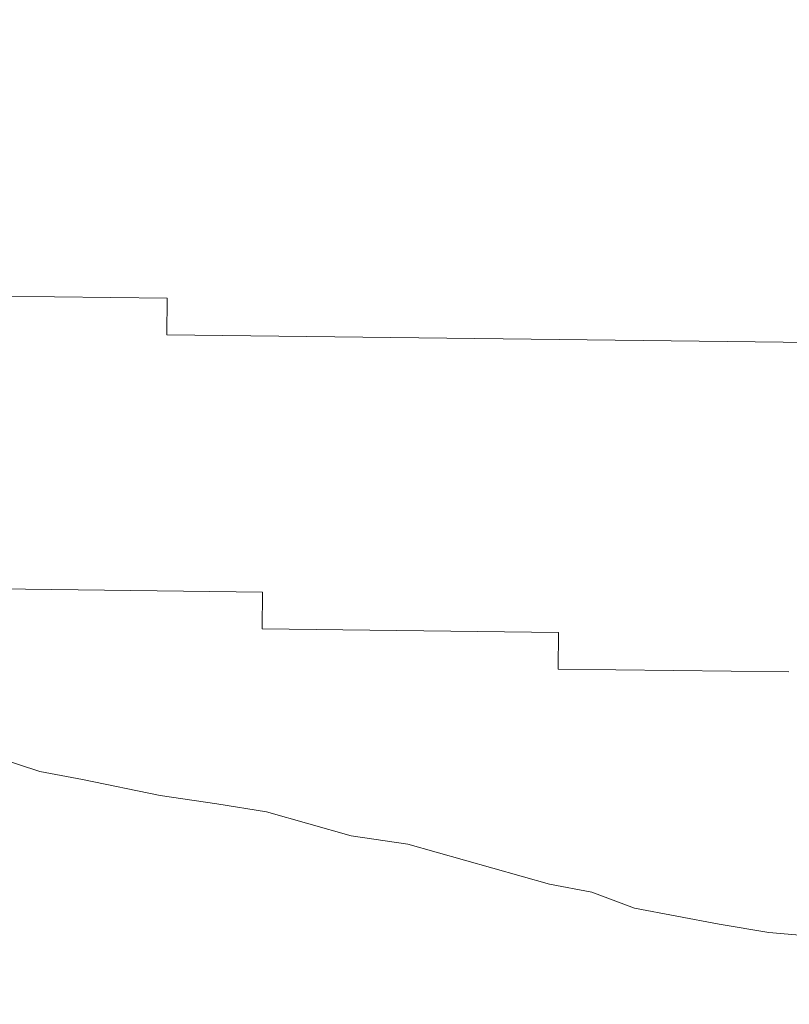
# Model space of a CAD drawing. Units: inches. Extents: x -466983 to 1020, y 324 to 318697.
# Tile 57 of 97: x 637.858 to 640.764, y 938.98 to 942.694. Entities that reach past the tile are written whole.
import ezdxf

# ---------------------------------------------------------------- set-up
doc = ezdxf.new("R2010")
doc.units = ezdxf.units.IN
doc.header["$MEASUREMENT"] = 0
doc.layers.add('A-FLOR-PATT', color=252, linetype='Continuous', lineweight=13)
doc.layers.add('A-FURN', color=8, linetype='Continuous', lineweight=18)

# ---------------------------------------------------------------- blocks, each defined once
blk = doc.blocks.new('L Shaped Sofa')
at = {"ltscale": 2}
for p, q in [((2423.7715, 750.0772), (2424.4056, 750.02)), ((2424.4056, 750.02), (2424.7468, 749.9642)), ((2424.7468, 749.9642), (2425.3317, 749.853)), ((2425.3317, 749.853), (2425.6238, 749.7432)), ((2425.6238, 749.7432), (2425.9162, 749.6876)), ((2425.9162, 749.6876), (2426.8905, 749.412)), ((2426.8905, 749.412), (2427.2805, 749.3559)), ((2427.2805, 749.3559), (2427.865, 749.1905)), ((2427.865, 749.1905), (2428.2063, 749.1347)), ((2428.2063, 749.1347), (2428.5963, 749.0787)), ((2428.5963, 749.0787), (2429.1324, 748.9677)), ((2429.1324, 748.9677), (2429.4248, 748.9121)), ((2429.4248, 748.9121), (2429.7657, 748.8021)), ((2424.2687, 748.2269), (2425.8566, 748.2075)), ((2425.8566, 748.2075), (2425.8535, 747.9556)), ((2425.8535, 747.9556), (2427.895, 747.9306)), ((2427.895, 747.9306), (2427.8919, 747.6787)), ((2427.8919, 747.6787), (2429.7066, 747.6565)), ((2423.3337, 745.9707), (2428.5509, 745.907)), ((2428.5509, 745.907), (2428.5478, 745.6551)), ((2428.5478, 745.6551), (2430.8162, 745.6274))]:
    blk.add_line(p, q, dxfattribs=at)

msp = doc.modelspace()

# ---------------------------------------------------------------- hatches: boundary and pattern name
at = {"layer": 'A-FLOR-PATT', "transparency": 33554572}
h = msp.add_hatch(dxfattribs=at)
h.set_pattern_fill('ANSI37', color=256, scale=30)
h.set_pattern_definition([(45, (-1212.4137, -290.035), (-2.6516504, 2.6516504), []), (135, (-1212.4137, -290.035), (-2.6516504, -2.6516504), [])])
h.paths.add_polyline_path([(901.8057, 1075.9377), (900.6144, 1075.9377), (900.6144, 1065.3856), (899.391, 1065.3856), (898.0911, 1065.3856), (892.8356, 1058.7098, -0.258377), (892.1875, 1058.3509), (879.9848, 1058.3509, -0.20177), (879.4382, 1058.5808), (874.0812, 1065.3856), (872.7813, 1065.3856), (871.5579, 1065.3856), (871.5579, 1075.9377), (813.8057, 1075.9377), (813.8057, 1044.7922), (832.3947, 1044.7922, -0.394795), (848.6602, 1028.5356), (848.6602, 1009.9377), (901.8057, 1009.9377), (901.8057, 1015.9377), (901.3057, 1015.9377), (871.3057, 1015.9377), (871.3057, 1017.2502), (871.3344, 1017.2502, -0.401453), (901.3057, 1045.9377), (901.8057, 1045.9377)])
edge = h.paths.add_edge_path(flags=16)
edge.add_line((847.7731, 1068.9486), (847.7731, 1073.7088))
edge.add_arc((849.2269, 1073.7088), 1.4538, 90, 180, ccw=False)
edge.add_line((849.2269, 1075.1627), (864.4921, 1075.1627))
edge.add_arc((864.4921, 1073.7088), 1.4538, 0, 90, ccw=False)
edge.add_line((865.9459, 1073.7088), (865.9459, 1069.0035))
edge.add_arc((832.6447, 1068.9761), 33.3012, -20.61234, 0.04725, ccw=False)
edge.add_ellipse((856.8595, 1058.48), major_axis=(0, 10.2131), ratio=0.6859192, start_angle=100.00884, end_angle=259.99116, ccw=False)
edge.add_arc((881.0742, 1068.9761), 33.3012, 180.04725, 200.61234, ccw=False)
h.paths.add_polyline_path([(853.1456, 1066.4815), (853.1456, 1066.4534), (853.1463, 1066.4534, 0.433107), (852.9166, 1066.6849), (852.9166, 1066.4534), (853.1456, 1066.4534), (853.1456, 1066.4815), (853.088, 1066.6122, 0.697939), (852.6995, 1066.4534), (852.7003, 1066.4534), (852.7003, 1066.4815), (852.9166, 1067.0012), (852.9166, 1066.6849, -0.396254)], flags=0)
h.paths.add_polyline_path([(861.0187, 1066.4815), (861.0187, 1066.4534), (861.0194, 1066.4534, 0.416404), (860.8024, 1066.6849), (860.8024, 1066.4534), (861.0187, 1066.4534), (861.0187, 1066.4815), (860.9672, 1066.6053, 0.713344), (860.5726, 1066.4534), (860.5734, 1066.4534), (860.5734, 1066.4815), (860.8024, 1067.0012), (860.8024, 1066.6849, -0.379973)], flags=0)
edge = h.paths.add_edge_path(flags=0)
edge.add_spline(control_points=[(861.1298, 1065.7855), (861.4661, 1065.2478), (861.6134, 1065.0161), (861.9833, 1064.3736), (862.1924, 1063.9443), (862.5614, 1063.0391), (862.7212, 1062.5633), (862.9865, 1061.5781), (863.092, 1061.0689), (863.2452, 1060.031), (863.293, 1059.5025), (863.3295, 1058.4409), (863.3181, 1057.9078), (863.2366, 1056.8518), (863.1664, 1056.3289), (862.9695, 1055.308), (862.8427, 1054.8099), (862.5365, 1053.8522), (862.3571, 1053.3927), (861.9514, 1052.5249), (861.7251, 1052.1166), (861.233, 1051.3622), (860.9672, 1051.0162), (860.4048, 1050.3949), (860.1082, 1050.1197), (859.4937, 1049.6461), (859.1758, 1049.4476), (858.5276, 1049.1299), (858.1973, 1049.0107), (857.5315, 1048.8518), (857.1959, 1048.8121), (856.5249, 1048.812), (856.1894, 1048.8515), (855.5236, 1049.0101), (855.1933, 1049.1291), (854.545, 1049.4465), (854.2271, 1049.6449), (853.6124, 1050.1183), (853.3158, 1050.3933), (852.7533, 1051.0143), (852.4874, 1051.3602), (851.9952, 1052.1144), (851.7688, 1052.5225), (851.3629, 1053.3902), (851.1834, 1053.8496), (850.877, 1054.8071), (850.7501, 1055.3051), (850.553, 1056.326), (850.4827, 1056.8488), (850.401, 1057.9048), (850.3895, 1058.4379), (850.4257, 1059.4995), (850.4734, 1060.0281), (850.6265, 1061.066), (850.7318, 1061.5753), (850.9969, 1062.5605), (851.1567, 1063.0365), (851.5254, 1063.9418), (851.7345, 1064.3712), (852.1056, 1065.0164), (852.2544, 1065.2503), (852.6082, 1065.7335)], knot_values=[3.915332, 3.915332, 3.915332, 3.915332, 4.013468, 4.013468, 4.175532, 4.175532, 4.337596, 4.337596, 4.49966, 4.49966, 4.661724, 4.661724, 4.823788, 4.823788, 4.985852, 4.985852, 5.147916, 5.147916, 5.30998, 5.30998, 5.472044, 5.472044, 5.634109, 5.634109, 5.796173, 5.796173, 5.958237, 5.958237, 6.120301, 6.120301, 6.282365, 6.282365, 6.444429, 6.444429, 6.606493, 6.606493, 6.768557, 6.768557, 6.930621, 6.930621, 7.092685, 7.092685, 7.254749, 7.254749, 7.416813, 7.416813, 7.578878, 7.578878, 7.740942, 7.740942, 7.903006, 7.903006, 8.06507, 8.06507, 8.227134, 8.227134, 8.389198, 8.389198, 8.551262, 8.551262, 8.65037, 8.65037, 8.65037, 8.65037], degree=3, periodic=0)
edge.add_line((852.6421, 1065.7855), (861.1298, 1065.7855))
edge = h.paths.add_edge_path(flags=0)
edge.add_ellipse((856.8496, 1057.7432), major_axis=(0, 7.7921), ratio=0.687861, start_angle=0, end_angle=360)
h.paths.add_polyline_path([(848.8634, 1069.3891), (848.8634, 1073.9605, -0.414214), (849.9538, 1075.0508), (863.7652, 1075.0508, -0.414214), (864.8555, 1073.9605), (864.8555, 1069.3891, -0.388936), (864.5237, 1069.027, -0.043561), (849.1953, 1069.027, -0.388936)], flags=0)
h.paths.add_polyline_path([(853.1006, 1068.1122, -1), (852.6775, 1068.1122, -1)], flags=0)
edge = h.paths.add_edge_path(flags=0)
edge.add_ellipse((856.8595, 1057.3378), major_axis=(0, 2.207), ratio=0.657164, start_angle=0, end_angle=360)
h.paths.add_polyline_path([(861.0415, 1068.1122, -1), (860.6184, 1068.1122, -1)], flags=0)
edge = h.paths.add_edge_path()
edge.add_line((573.9537, 1057.3412), (573.9537, 1075.9377))
edge.add_line((573.9537, 1075.9377), (558.7308, 1075.9377))
edge.add_line((558.7308, 1075.9377), (558.7308, 1065.3856))
edge.add_line((558.7308, 1065.3856), (557.5074, 1065.3856))
edge.add_line((557.5074, 1065.3856), (556.2075, 1065.3856))
edge.add_line((556.2075, 1065.3856), (550.952, 1058.7098))
edge.add_arc((550.3039, 1059.1155), 0.7646, 270, 327.9483, ccw=False)
edge.add_line((550.3039, 1058.3509), (538.1012, 1058.3509))
edge.add_arc((538.1012, 1059.1155), 0.7646, 224.3704, 270, ccw=False)
edge.add_line((537.5546, 1058.5808), (532.1976, 1065.3856))
edge.add_line((532.1976, 1065.3856), (530.8977, 1065.3856))
edge.add_line((530.8977, 1065.3856), (529.6743, 1065.3856))
edge.add_line((529.6743, 1065.3856), (529.6743, 1075.9377))
edge.add_line((529.6743, 1075.9377), (520.8057, 1075.9377))
edge.add_line((520.8057, 1075.9377), (520.8057, 1045.9377))
edge.add_line((520.8057, 1045.9377), (521.3057, 1045.9377))
edge.add_arc((521.3057, 1015.9377), 30, 2.50749, 90, ccw=False)
edge.add_line((551.277, 1017.2502), (551.3057, 1017.2502))
edge.add_line((551.3057, 1017.2502), (551.3057, 1015.9377))
edge.add_line((551.3057, 1015.9377), (520.8057, 1015.9377))
edge.add_line((520.8057, 1015.9377), (520.8057, 1009.9377))
edge.add_line((520.8057, 1009.9377), (559.1913, 1010.4022))
edge.add_arc((559.1913, 1011.856), 1.4538, 180, 270, ccw=False)
edge.add_line((557.7375, 1011.856), (557.7375, 1016.5613))
edge.add_arc((591.0386, 1016.5888), 33.3012, 159.38766, 180.04725, ccw=False)
edge.add_ellipse((566.8239, 1027.0848), major_axis=(0, 10.2131), ratio=0.6859192, start_angle=280.00884, end_angle=439.99116, ccw=False)
edge.add_arc((542.6091, 1016.5888), 33.3012, 0.04725, 20.61234, ccw=False)
edge.add_line((575.9103, 1016.6162), (575.9103, 1011.856))
edge.add_arc((574.4565, 1011.856), 1.4538, -90, 0, ccw=False)
edge.add_line((574.4565, 1010.4022), (608.8057, 1009.9377))
edge.add_line((608.8057, 1009.9377), (608.8057, 1041.0857))
edge.add_line((608.8057, 1041.0857), (590.2179, 1041.0857))
edge.add_arc((590.775, 1057.9074), 16.8309, 181.92775, 268.10321, ccw=False)
edge = h.paths.add_edge_path()
edge.add_ellipse((494.2443, 583.6204), major_axis=(0, 10.2131), ratio=0.6859192, start_angle=280.00884, end_angle=439.99116, ccw=False)
edge.add_arc((470.0296, 573.1243), 33.3012, 0.04725, 20.61234, ccw=False)
edge.add_line((503.3307, 573.1518), (503.3307, 568.3916))
edge.add_arc((501.8769, 568.3916), 1.4538, -90, 0, ccw=False)
edge.add_line((501.8769, 566.9377), (539.8057, 566.9377))
edge.add_line((539.8057, 566.9377), (539.8057, 572.9377))
edge.add_line((539.8057, 572.9377), (539.3057, 572.9377))
edge.add_line((539.3057, 572.9377), (509.3057, 572.9377))
edge.add_line((509.3057, 572.9377), (509.3057, 574.2502))
edge.add_line((509.3057, 574.2502), (509.3344, 574.2502))
edge.add_arc((539.3057, 572.9377), 30, 90, 177.49251, ccw=False)
edge.add_line((539.3057, 602.9377), (539.8057, 602.9377))
edge.add_line((539.8057, 602.9377), (539.8057, 626.9377))
edge.add_line((539.8057, 626.9377), (531.7718, 626.9377))
edge.add_line((531.7718, 626.9377), (531.7718, 616.3856))
edge.add_line((531.7718, 616.3856), (530.5484, 616.3856))
edge.add_line((530.5484, 616.3856), (529.2485, 616.3856))
edge.add_line((529.2485, 616.3856), (523.7105, 609.3509))
edge.add_line((523.7105, 609.3509), (510.7766, 609.3509))
edge.add_line((510.7766, 609.3509), (505.2386, 616.3856))
edge.add_line((505.2386, 616.3856), (503.9387, 616.3856))
edge.add_line((503.9387, 616.3856), (502.7153, 616.3856))
edge.add_line((502.7153, 616.3856), (502.7153, 626.9377))
edge.add_line((502.7153, 626.9377), (481.6983, 626.9377))
edge.add_line((481.6983, 626.9377), (481.6983, 610.995))
edge.add_arc((467.2703, 611.4728), 14.4359, 271.92775, 358.10321, ccw=False)
edge.add_line((467.7559, 597.0451), (451.8057, 597.0451))
edge.add_line((451.8057, 597.0451), (451.8057, 584.4035))
edge.add_line((451.8057, 584.4035), (451.8057, 566.9377))
edge.add_line((451.8057, 566.9377), (486.6117, 566.9377))
edge.add_arc((486.6117, 568.3916), 1.4538, 180, 270, ccw=False)
edge.add_line((485.1579, 568.3916), (485.1579, 573.0969))
edge.add_arc((518.4591, 573.1243), 33.3012, 159.38766, 180.04725, ccw=False)
h.paths.add_polyline_path([(836.2609, 1020.7328), (879.8898, 1020.7328), (879.8898, 1039.3902), (836.2609, 1039.3902)], flags=25)
h.paths.add_polyline_path([(549.9851, 1036.7492), (593.614, 1036.7492), (593.614, 1055.4065), (549.9851, 1055.4065)], flags=24)
h.paths.add_polyline_path([(475.123, 595.5959), (518.752, 595.5959), (518.752, 614.2532), (475.123, 614.2532)], flags=24)
h = msp.add_hatch(dxfattribs=at)
h.set_pattern_fill('ANSI37', color=256, scale=20)
h.set_pattern_definition([(45, (-1212.4137, -290.035), (-1.767767, 1.767767), []), (135, (-1212.4137, -290.035), (-1.767767, -1.767767), [])])
h.paths.add_polyline_path([(809.8057, 870.9377), (809.8057, 888.1519), (806.9985, 888.1519), (802.6624, 888.1519), (789.3832, 888.1519), (786.2846, 888.1519, -0.414214), (785.4991, 888.9374), (785.4991, 900.1959), (785.4991, 908.4696, -0.414214), (786.8082, 909.7787, -0.414214), (785.4991, 911.0878), (785.4991, 929.1015, -0.414214), (786.8082, 930.4106, -0.414214), (785.4991, 931.7197), (785.4991, 931.9039, -0.414214), (784.19, 930.5948), (766.7223, 930.5948, -0.412359), (765.4132, 931.8956, -0.413741), (764.1145, 930.5782), (744.5781, 930.422, -0.416556), (743.7864, 931.2075), (743.7864, 933.5153), (742.2154, 933.5153), (742.2154, 952.024, -0.001344), (743.7864, 952.1998), (743.7864, 953.9377), (678.5915, 953.9377), (678.5915, 951.1305), (678.5915, 946.7945), (678.5915, 933.5153), (678.5915, 930.4166, -0.414214), (677.806, 929.6312), (666.5475, 929.6312), (658.2738, 929.6312, -0.414214), (656.9647, 930.9403, -0.414214), (655.6556, 929.6312), (637.6419, 929.6312, -0.414214), (636.3328, 930.9403, -0.414214), (635.0237, 929.6312), (634.8395, 929.6312, -0.414214), (636.1486, 928.322), (636.1486, 910.8544, -0.412359), (634.8478, 909.5452, -0.413741), (636.1653, 908.2466), (636.3214, 888.7102, -0.416556), (635.5359, 887.9184), (633.2281, 887.9184), (633.2281, 886.3475), (614.7194, 886.3475, -0.001344), (614.5436, 887.9184), (612.8057, 887.9184), (612.8057, 834.9377), (612.8057, 752.9377), (612.8057, 748.9377), (612.8057, 697.9377), (654.8057, 697.9377), (654.8057, 701.9377), (715.8057, 701.9377), (715.8057, 737.4353), (774.2918, 737.4353), (774.2918, 795.9377), (809.8057, 795.9377)])
h.paths.add_polyline_path([(679.2761, 849.5757, 0.102523), (682.1475, 849.2608, -0.080461), (694.5428, 849.7725, -0.283899), (694.4822, 849.0082, 0.136605), (694.4068, 848.8103, -0.030441), (694.5428, 846.8929), (694.5428, 842.6198), (694.5428, 838.3466, -0.028219), (694.4246, 836.5684), (694.425, 836.5684, 0.196187), (694.4456, 836.2708, -0.302897), (694.5428, 835.467, -0.080461), (682.1475, 835.9787, 0.102523), (679.2761, 835.6638, -0.58611), (678.6457, 836.0169), (678.6457, 849.2227, -0.58611)], flags=16)
h.paths.add_polyline_path([(679.5173, 848.6515, 0.699597), (679.476, 848.6342, 1.20716), (679.1935, 848.7422, 0.010621)], flags=0)
h.paths.add_polyline_path([(679.4923, 836.5608, -0.013798), (679.9178, 836.6594, -0.071703), (682.8533, 837.1434, -0.165743), (682.1665, 839.1006), (682.1665, 842.6094), (682.1665, 846.0603, -0.240616), (683.4733, 848.6767, -0.068263), (693.9295, 849.0082), (693.7875, 848.7083), (693.7875, 849.0228, 0.067332), (683.4733, 848.6767, 0.240616), (682.1665, 846.0603), (682.1665, 842.6094), (682.1665, 839.1006, 0.23459), (683.461, 836.5513, 0.068093), (693.7875, 836.1955), (693.7875, 836.5104), (693.9296, 836.2102, -0.077215), (682.2421, 836.7815, 0.086627), (679.5283, 836.5701, -0.628402), (679.5029, 836.5735), (679.5029, 836.6071, 0.910458)], flags=0)
h.paths.add_polyline_path([(679.476, 848.6364), (679.2069, 848.647), (679.2069, 836.5718, 0.913566), (679.3645, 836.5861), (679.476, 836.5824)], flags=0)
h.paths.add_polyline_path([(679.2761, 829.8604, 0.102523), (682.1475, 829.5455, -0.080461), (694.5428, 830.0572, -0.283899), (694.4822, 829.2929, 0.136605), (694.4068, 829.095, -0.030441), (694.5428, 827.1776), (694.5428, 822.9045), (694.5428, 818.6314, -0.028219), (694.4246, 816.8531), (694.425, 816.8532, 0.196187), (694.4456, 816.5555, -0.302897), (694.5428, 815.7517, -0.080461), (682.1475, 816.2635, 0.102523), (679.2761, 815.9485, -0.58611), (678.6457, 816.3016), (678.6457, 829.5074, -0.58611)], flags=16)
h.paths.add_polyline_path([(679.5173, 828.9362, 0.699597), (679.476, 828.9189, 1.20716), (679.1935, 829.0269, 0.010621)], flags=0)
h.paths.add_polyline_path([(679.4923, 816.8456, -0.013798), (679.9178, 816.9441, -0.071703), (682.8533, 817.4281, -0.165743), (682.1665, 819.3853), (682.1665, 822.8941), (682.1665, 826.345, -0.240616), (683.4733, 828.9614, -0.068263), (693.9295, 829.2929), (693.7875, 828.9931), (693.7875, 829.3076, 0.067332), (683.4733, 828.9614, 0.240616), (682.1665, 826.345), (682.1665, 822.8941), (682.1665, 819.3853, 0.23459), (683.461, 816.836, 0.068093), (693.7875, 816.4802), (693.7875, 816.7952), (693.9296, 816.4949, -0.077215), (682.2421, 817.0662, 0.086627), (679.5283, 816.8549, -0.628402), (679.5029, 816.8582), (679.5029, 816.8918, 0.910458)], flags=0)
h.paths.add_polyline_path([(679.476, 828.9211), (679.2069, 828.9317), (679.2069, 816.8565, 0.913566), (679.3645, 816.8708), (679.476, 816.8671)], flags=0)
h.paths.add_polyline_path([(679.2761, 810.1451, 0.102523), (682.1475, 809.8302, -0.080461), (694.5428, 810.342, -0.3023), (694.4466, 809.5394, 0.10023), (694.4058, 809.3878, -0.03057), (694.5428, 807.4623), (694.5428, 803.1892), (694.5428, 798.9161, -0.03057), (694.4058, 796.9906, 0.10023), (694.4466, 796.839, -0.3023), (694.5428, 796.0365, -0.080461), (682.1475, 796.5482, 0.102523), (679.2761, 796.2333, -0.58611), (678.6457, 796.5863), (678.6457, 809.7921, -0.58611)], flags=16)
h.paths.add_polyline_path([(679.5173, 809.2417, 0.699597), (679.476, 809.2244, 1.20716), (679.1935, 809.3324, 0.010621)], flags=0)
h.paths.add_polyline_path([(679.4923, 797.151, -0.013798), (679.9178, 797.2496, -0.071703), (682.8533, 797.7336, -0.165743), (682.1665, 799.6908), (682.1665, 803.1996), (682.1665, 806.6505, -0.239349), (683.461, 809.2577, -0.072465), (694.4468, 809.5405, 0.197932), (694.425, 809.2405), (693.7875, 809.2985), (693.7875, 809.6135, 0.068093), (683.461, 809.2577, 0.239349), (682.1665, 806.6505), (682.1665, 803.1996), (682.1665, 799.6908, 0.235854), (683.4733, 797.1323, 0.067332), (693.7875, 796.7861), (693.7875, 797.1006), (694.425, 797.1586, 0.197932), (694.4468, 796.8586, -0.080419), (682.1557, 797.3795, 0.083867), (679.5283, 797.1603, -0.628402), (679.5029, 797.1637), (679.5029, 797.1973, 0.910458)], flags=0)
h.paths.add_polyline_path([(679.2069, 809.2372), (679.2069, 797.162, 0.913566), (679.3645, 797.1763), (679.476, 797.1726), (679.476, 809.2266)], flags=0)
h.paths.add_polyline_path([(695.3643, 853.2989), (728.2231, 853.2989), (728.2231, 771.1519), (695.3643, 771.1519)], flags=16)
h.paths.add_polyline_path([(696.0215, 852.6417), (727.5659, 852.6417), (727.5659, 771.809), (696.0215, 771.809)], flags=0)
h.paths.add_polyline_path([(679.2761, 788.7869, 0.102523), (682.1475, 788.472, -0.080461), (694.5428, 788.9837, -0.3023), (694.4466, 788.1812, 0.10023), (694.4058, 788.0296, -0.03057), (694.5428, 786.1041), (694.5428, 781.831), (694.5428, 777.5578, -0.03057), (694.4058, 775.6323, 0.10023), (694.4466, 775.4808, -0.3023), (694.5428, 774.6782, -0.080461), (682.1475, 775.19, 0.102523), (679.2761, 774.875, -0.58611), (678.6457, 775.2281), (678.6457, 788.4339, -0.58611)], flags=16)
h.paths.add_polyline_path([(679.5173, 787.8834, 0.699597), (679.476, 787.8662, 1.20716), (679.1935, 787.9742, 0.010621)], flags=0)
h.paths.add_polyline_path([(679.4923, 775.7928, -0.013798), (679.9178, 775.8914, -0.071703), (682.8533, 776.3753, -0.165743), (682.1665, 778.3325), (682.1665, 781.8414), (682.1665, 785.2922, -0.239349), (683.461, 787.8995, -0.072465), (694.4468, 788.1823, 0.197932), (694.425, 787.8823), (693.7875, 787.9403), (693.7875, 788.2553, 0.068093), (683.461, 787.8995, 0.239349), (682.1665, 785.2922), (682.1665, 781.8414), (682.1665, 778.3325, 0.235854), (683.4733, 775.7741, 0.067332), (693.7875, 775.4279), (693.7875, 775.7424), (694.425, 775.8004, 0.197932), (694.4468, 775.5004, -0.080419), (682.1557, 776.0212, 0.083867), (679.5283, 775.8021, -0.628402), (679.5029, 775.8054), (679.5029, 775.8391, 0.910458)], flags=0)
h.paths.add_polyline_path([(679.2069, 787.8789), (679.2069, 775.8038, 0.913566), (679.3645, 775.818), (679.476, 775.8144), (679.476, 787.8684)], flags=0)
h.paths.add_polyline_path([(704.641, 854.1204, -0.080461), (705.1527, 866.5157, 0.102523), (704.8378, 869.3871, -0.58611), (705.1908, 870.0174), (718.3966, 870.0174, -0.58611), (718.7496, 869.3871, 0.102523), (718.4347, 866.5157, -0.080461), (718.9465, 854.1204, -0.3023), (718.1439, 854.2166, 0.10023), (717.9924, 854.2574, -0.03057), (716.0668, 854.1204), (711.7937, 854.1204), (707.5206, 854.1204, -0.03057), (705.5951, 854.2574, 0.10023), (705.4435, 854.2166, -0.3023)], flags=16)
h.paths.add_polyline_path([(717.8462, 869.1459, 0.699597), (717.8289, 869.1872, 1.20716), (717.9369, 869.4697, 0.010621)], flags=0)
h.paths.add_polyline_path([(705.4631, 854.2164, -0.080419), (705.984, 866.5074, 0.083867), (705.7648, 869.1349, -0.628402), (705.7682, 869.1603), (705.8018, 869.1603, 0.910458), (705.7555, 869.1709, -0.013798), (705.8541, 868.7454, -0.071703), (706.3381, 865.8099, -0.165743), (708.2953, 866.4967), (711.8041, 866.4967), (715.255, 866.4967, -0.239349), (717.8622, 865.2022, -0.072465), (718.145, 854.2164, 0.197932), (717.845, 854.2382), (717.903, 854.8757), (718.218, 854.8757, 0.068093), (717.8622, 865.2022, 0.239349), (715.255, 866.4967), (711.8041, 866.4967), (708.2953, 866.4967, 0.235854), (705.7368, 865.1898, 0.067332), (705.3906, 854.8757), (705.7051, 854.8757), (705.7631, 854.2382, 0.197932)], flags=16)
h.paths.add_polyline_path([(705.7665, 869.4563, 0.913566), (705.7808, 869.2987), (705.7771, 869.1872), (717.8311, 869.1872), (717.8417, 869.4563)], flags=0)
h.paths.add_polyline_path([(729.0446, 842.6198), (729.0446, 846.8929, -0.03057), (729.1817, 848.8184, 0.10023), (729.1408, 848.9699, -0.3023), (729.0446, 849.7725, -0.080461), (741.4399, 849.2608, 0.102523), (744.3113, 849.5757, -0.58611), (744.9417, 849.2227), (744.9417, 836.0169, -0.58611), (744.3113, 835.6638, 0.102523), (741.4399, 835.9787, -0.080461), (729.0446, 835.467, -0.3023), (729.1408, 836.2696, 0.10023), (729.1817, 836.4211, -0.03057), (729.0446, 838.3466)], flags=16)
h.paths.add_polyline_path([(744.1115, 836.5846, 1.20716), (744.3939, 836.4766, 0.010621), (744.0701, 836.5673, 0.699597)], flags=0)
h.paths.add_polyline_path([(729.1407, 836.2684, 0.197932), (729.1624, 836.5684), (729.7999, 836.5104), (729.7999, 836.1955, 0.068093), (740.1264, 836.5513, 0.239349), (741.4209, 839.1585), (741.4209, 842.6094), (741.4209, 846.1182, 0.235854), (740.1141, 848.6767, 0.067332), (729.7999, 849.0228), (729.7999, 848.7083), (729.1624, 848.6503, 0.197932), (729.1407, 848.9504, -0.080419), (741.4317, 848.4295, 0.083867), (744.0591, 848.6486, -0.628402), (744.0845, 848.6453), (744.0845, 848.6117, 0.910458), (744.0951, 848.6579, -0.013798), (743.6696, 848.5594, -0.071703), (740.7341, 848.0754, -0.165743), (741.4209, 846.1182), (741.4209, 842.6094), (741.4209, 839.1585, -0.239349), (740.1264, 836.5513, -0.072465)], flags=0)
h.paths.add_polyline_path([(729.0446, 830.0572, -0.080461), (741.4399, 829.5455, 0.102523), (744.3113, 829.8604, -0.58611), (744.9417, 829.5074), (744.9417, 816.3016, -0.58611), (744.3113, 815.9485, 0.102523), (741.4399, 816.2635, -0.080461), (729.0446, 815.7517, -0.3023), (729.1408, 816.5543, 0.10023), (729.1817, 816.7058, -0.03057), (729.0446, 818.6314), (729.0446, 822.9045), (729.0446, 827.1776, -0.03057), (729.1817, 829.1031, 0.10023), (729.1408, 829.2547, -0.3023)], flags=16)
h.paths.add_polyline_path([(744.1115, 816.8693, 1.20716), (744.3939, 816.7613, 0.010621), (744.0701, 816.852, 0.699597)], flags=0)
h.paths.add_polyline_path([(729.1407, 829.2351, -0.080419), (741.4317, 828.7142, 0.083867), (744.0591, 828.9334, -0.628402), (744.0845, 828.93), (744.0845, 828.8964, 0.910458), (744.0951, 828.9427, -0.013798), (743.6696, 828.8441, -0.071703), (740.7341, 828.3601, -0.165743), (741.4209, 826.4029), (741.4209, 822.8941), (741.4209, 819.4432, -0.239349), (740.1264, 816.836, -0.072465), (729.1407, 816.5531, 0.197932), (729.1624, 816.8532), (729.7999, 816.7952), (729.7999, 816.4802, 0.068093), (740.1264, 816.836, 0.239349), (741.4209, 819.4432), (741.4209, 822.8941), (741.4209, 826.4029, 0.235854), (740.1141, 828.9614, 0.067332), (729.7999, 829.3076), (729.7999, 828.9931), (729.1624, 828.9351, 0.197932)], flags=16)
h.paths.add_polyline_path([(729.0446, 810.342, -0.080461), (741.4399, 809.8302, 0.102523), (744.3113, 810.1451, -0.58611), (744.9417, 809.7921), (744.9417, 796.5863, -0.58611), (744.3113, 796.2333, 0.102523), (741.4399, 796.5482, -0.080461), (729.0446, 796.0365, -0.283899), (729.1052, 796.8007, 0.136605), (729.1806, 796.9987, -0.030441), (729.0446, 798.9161), (729.0446, 803.1892), (729.0446, 807.4623, -0.028219), (729.1628, 809.2406), (729.1624, 809.2405, 0.196187), (729.1418, 809.5382, -0.302897)], flags=16)
h.paths.add_polyline_path([(744.1115, 797.1748, 1.20716), (744.3939, 797.0668, 0.010621), (744.0701, 797.1575, 0.699597)], flags=0)
h.paths.add_polyline_path([(741.3453, 809.0275, 0.086627), (744.0591, 809.2388, -0.628402), (744.0845, 809.2355), (744.0845, 809.2019, 0.910458), (744.0951, 809.2481, -0.013798), (743.6696, 809.1496, -0.071703), (740.7341, 808.6656, -0.165743), (741.4209, 806.7084), (741.4209, 803.1996), (741.4209, 799.7487, -0.240616), (740.1141, 797.1323, -0.068263), (729.658, 796.8008), (729.7999, 797.1006), (729.7999, 796.7861, 0.067332), (740.1141, 797.1323, 0.240616), (741.4209, 799.7487), (741.4209, 803.1996), (741.4209, 806.7084, 0.23459), (740.1264, 809.2577, 0.068093), (729.7999, 809.6135), (729.7999, 809.2985), (729.6578, 809.5988, -0.077215)], flags=0)
h.paths.add_polyline_path([(704.641, 770.3304, -0.283899), (705.4053, 770.2697, 0.136605), (705.6032, 770.1944, -0.030441), (707.5206, 770.3304), (711.7937, 770.3304), (716.0668, 770.3304, -0.028219), (717.8451, 770.2122), (717.845, 770.2126, 0.196187), (718.1427, 770.2331, -0.302897), (718.9465, 770.3304, -0.080461), (718.4347, 757.9351, 0.102523), (718.7496, 755.0637, -0.58611), (718.3966, 754.4333), (705.1908, 754.4333, -0.58611), (704.8378, 755.0637, 0.102523), (705.1527, 757.9351, -0.080461)], flags=16)
h.paths.add_polyline_path([(705.762, 755.3048, 0.699597), (705.7793, 755.2635, 1.20716), (705.6713, 754.9811, 0.010621)], flags=0)
h.paths.add_polyline_path([(705.4053, 769.717), (705.7051, 769.5751), (705.3906, 769.5751, 0.067332), (705.7368, 759.2609, 0.240616), (708.3532, 757.954), (711.8041, 757.954), (715.3129, 757.954, 0.23459), (717.8622, 759.2485, 0.068093), (718.218, 769.5751), (717.903, 769.5751), (718.2033, 769.7172, -0.077215), (717.632, 758.0297, 0.086627), (717.8433, 755.3159, -0.628402), (717.84, 755.2904), (717.8064, 755.2904, 0.910458), (717.8526, 755.2799, -0.013798), (717.7541, 755.7053, -0.071703), (717.2701, 758.6409, -0.165743), (715.3129, 757.954), (711.8041, 757.954), (708.3532, 757.954, -0.240616), (705.7368, 759.2609, -0.068263)], flags=0)
h.paths.add_polyline_path([(729.0446, 788.9837, -0.080461), (741.4399, 788.472, 0.102523), (744.3113, 788.7869, -0.58611), (744.9417, 788.4339), (744.9417, 775.2281, -0.58611), (744.3113, 774.875, 0.102523), (741.4399, 775.19, -0.080461), (729.0446, 774.6782, -0.283899), (729.1052, 775.4425, 0.136605), (729.1806, 775.6405, -0.030441), (729.0446, 777.5578), (729.0446, 781.831), (729.0446, 786.1041, -0.028219), (729.1628, 787.8823), (729.1624, 787.8823, 0.196187), (729.1418, 788.1799, -0.302897)], flags=16)
h.paths.add_polyline_path([(744.1115, 775.8165, 1.20716), (744.3939, 775.7086, 0.010621), (744.0701, 775.7993, 0.699597)], flags=0)
h.paths.add_polyline_path([(741.3453, 787.6692, 0.086627), (744.0591, 787.8806, -0.628402), (744.0845, 787.8773), (744.0845, 787.8437, 0.910458), (744.0951, 787.8899, -0.013798), (743.6696, 787.7913, -0.071703), (740.7341, 787.3074, -0.165743), (741.4209, 785.3502), (741.4209, 781.8414), (741.4209, 778.3905, -0.240616), (740.1141, 775.7741, -0.068263), (729.658, 775.4425), (729.7999, 775.7424), (729.7999, 775.4279, 0.067332), (740.1141, 775.7741, 0.240616), (741.4209, 778.3905), (741.4209, 781.8414), (741.4209, 785.3502, 0.23459), (740.1264, 787.8995, 0.068093), (729.7999, 788.2553), (729.7999, 787.9403), (729.6578, 788.2405, -0.077215)], flags=0)
h.paths.add_polyline_path([(744.1115, 848.6364), (744.1115, 836.5824), (744.3805, 836.5718), (744.3805, 848.647, 0.913566), (744.2229, 848.6327)], flags=0)
h.paths.add_polyline_path([(744.2229, 828.9174), (744.1115, 828.9211), (744.1115, 816.8671), (744.3805, 816.8565), (744.3805, 828.9317, 0.913566)], flags=0)
h.paths.add_polyline_path([(717.8311, 755.2635), (705.7771, 755.2635), (705.7665, 754.9945), (717.8417, 754.9945, 0.913566), (717.8274, 755.1521)], flags=0)
h.paths.add_polyline_path([(744.2229, 809.2229), (744.1115, 809.2266), (744.1115, 797.1726), (744.3805, 797.162), (744.3805, 809.2372, 0.913566)], flags=0)
h.paths.add_polyline_path([(744.1115, 787.8684), (744.1115, 775.8144), (744.3805, 775.8038), (744.3805, 787.8789, 0.913566), (744.2229, 787.8647)], flags=0)
h.paths.add_polyline_path([(678.8774, 877.1228), (737.6127, 877.1228), (737.6127, 899.5116), (678.8774, 899.5116)], flags=24)

# ---------------------------------------------------------------- linework, layer by layer
at = {"layer": 'A-FURN', "ltscale": 2}
for p, q in [((638.4155, 941.6436), (637.172, 941.6588)), ((638.4155, 941.6436), (637.172, 941.6588)), ((638.4155, 941.6436), (637.172, 941.6588)), ((638.4155, 941.6436), (637.172, 941.6588)), ((638.4155, 941.6436), (637.172, 941.6588)), ((638.4155, 941.6436), (637.172, 941.6588)), ((638.4139, 941.5055), (638.4155, 941.6436)), ((638.4139, 941.5055), (638.4155, 941.6436)), ((638.4139, 941.5055), (638.4155, 941.6436)), ((638.4139, 941.5055), (638.4155, 941.6436)), ((638.4139, 941.5055), (638.4155, 941.6436)), ((638.4139, 941.5055), (638.4155, 941.6436)), ((641.274, 941.4706), (638.4139, 941.5055)), ((641.274, 941.4706), (638.4139, 941.5055)), ((641.274, 941.4706), (638.4139, 941.5055)), ((641.274, 941.4706), (638.4139, 941.5055)), ((641.274, 941.4706), (638.4139, 941.5055)), ((641.274, 941.4706), (638.4139, 941.5055)), ((638.7751, 940.5343), (637.7803, 940.5464)), ((638.7751, 940.5343), (637.7803, 940.5464)), ((638.7751, 940.5343), (637.7803, 940.5464)), ((638.7751, 940.5343), (637.7803, 940.5464)), ((638.7751, 940.5343), (637.7803, 940.5464)), ((638.7751, 940.5343), (637.7803, 940.5464)), ((638.7734, 940.3962), (638.7751, 940.5343)), ((638.7734, 940.3962), (638.7751, 940.5343)), ((638.7734, 940.3962), (638.7751, 940.5343)), ((638.7734, 940.3962), (638.7751, 940.5343)), ((638.7734, 940.3962), (638.7751, 940.5343)), ((638.7734, 940.3962), (638.7751, 940.5343)), ((639.8926, 940.3825), (638.7734, 940.3962)), ((639.8926, 940.3825), (638.7734, 940.3962)), ((639.8926, 940.3825), (638.7734, 940.3962)), ((639.8926, 940.3825), (638.7734, 940.3962)), ((639.8926, 940.3825), (638.7734, 940.3962)), ((639.8926, 940.3825), (638.7734, 940.3962)), ((639.8909, 940.2444), (639.8926, 940.3825)), ((639.8909, 940.2444), (639.8926, 940.3825)), ((639.8909, 940.2444), (639.8926, 940.3825)), ((639.8909, 940.2444), (639.8926, 940.3825)), ((639.8909, 940.2444), (639.8926, 940.3825)), ((639.8909, 940.2444), (639.8926, 940.3825)), ((640.7614, 940.2337), (639.8909, 940.2444)), ((640.7614, 940.2337), (639.8909, 940.2444)), ((640.7614, 940.2337), (639.8909, 940.2444)), ((640.7614, 940.2337), (639.8909, 940.2444)), ((640.7614, 940.2337), (639.8909, 940.2444)), ((640.7614, 940.2337), (639.8909, 940.2444)), ((637.9348, 939.8581), (637.7479, 939.9184)), ((637.9348, 939.8581), (637.7479, 939.9184)), ((637.9348, 939.8581), (637.7479, 939.9184)), ((637.9348, 939.8581), (637.7479, 939.9184)), ((637.9348, 939.8581), (637.7479, 939.9184)), ((637.9348, 939.8581), (637.7479, 939.9184)), ((638.0951, 939.8276), (637.9348, 939.8581)), ((638.0951, 939.8276), (637.9348, 939.8581)), ((638.0951, 939.8276), (637.9348, 939.8581)), ((638.0951, 939.8276), (637.9348, 939.8581)), ((638.0951, 939.8276), (637.9348, 939.8581)), ((638.0951, 939.8276), (637.9348, 939.8581)), ((638.389, 939.7668), (638.0951, 939.8276)), ((638.389, 939.7668), (638.0951, 939.8276)), ((638.389, 939.7668), (638.0951, 939.8276)), ((638.389, 939.7668), (638.0951, 939.8276)), ((638.389, 939.7668), (638.0951, 939.8276)), ((638.389, 939.7668), (638.0951, 939.8276)), ((638.6028, 939.736), (638.389, 939.7668)), ((638.6028, 939.736), (638.389, 939.7668)), ((638.6028, 939.736), (638.389, 939.7668)), ((638.6028, 939.736), (638.389, 939.7668)), ((638.6028, 939.736), (638.389, 939.7668)), ((638.6028, 939.736), (638.389, 939.7668)), ((638.7899, 939.7054), (638.6028, 939.736)), ((638.7899, 939.7054), (638.6028, 939.736)), ((638.7899, 939.7054), (638.6028, 939.736)), ((638.7899, 939.7054), (638.6028, 939.736)), ((638.7899, 939.7054), (638.6028, 939.736)), ((638.7899, 939.7054), (638.6028, 939.736)), ((639.1103, 939.6148), (638.7899, 939.7054)), ((639.1103, 939.6148), (638.7899, 939.7054)), ((639.1103, 939.6148), (638.7899, 939.7054)), ((639.1103, 939.6148), (638.7899, 939.7054)), ((639.1103, 939.6148), (638.7899, 939.7054)), ((639.1103, 939.6148), (638.7899, 939.7054)), ((639.3241, 939.584), (639.1103, 939.6148)), ((639.3241, 939.584), (639.1103, 939.6148)), ((639.3241, 939.584), (639.1103, 939.6148)), ((639.3241, 939.584), (639.1103, 939.6148)), ((639.3241, 939.584), (639.1103, 939.6148)), ((639.3241, 939.584), (639.1103, 939.6148)), ((639.8582, 939.4329), (639.3241, 939.584)), ((639.8582, 939.4329), (639.3241, 939.584)), ((639.8582, 939.4329), (639.3241, 939.584)), ((639.8582, 939.4329), (639.3241, 939.584)), ((639.8582, 939.4329), (639.3241, 939.584)), ((639.8582, 939.4329), (639.3241, 939.584)), ((640.0186, 939.4024), (639.8582, 939.4329)), ((640.0186, 939.4024), (639.8582, 939.4329)), ((640.0186, 939.4024), (639.8582, 939.4329)), ((640.0186, 939.4024), (639.8582, 939.4329)), ((640.0186, 939.4024), (639.8582, 939.4329)), ((640.0186, 939.4024), (639.8582, 939.4329)), ((640.1787, 939.3422), (640.0186, 939.4024)), ((640.1787, 939.3422), (640.0186, 939.4024)), ((640.1787, 939.3422), (640.0186, 939.4024)), ((640.1787, 939.3422), (640.0186, 939.4024)), ((640.1787, 939.3422), (640.0186, 939.4024)), ((640.1787, 939.3422), (640.0186, 939.4024)), ((640.4993, 939.2813), (640.1787, 939.3422)), ((640.4993, 939.2813), (640.1787, 939.3422)), ((640.4993, 939.2813), (640.1787, 939.3422)), ((640.4993, 939.2813), (640.1787, 939.3422)), ((640.4993, 939.2813), (640.1787, 939.3422)), ((640.4993, 939.2813), (640.1787, 939.3422)), ((640.6864, 939.2507), (640.4993, 939.2813)), ((640.6864, 939.2507), (640.4993, 939.2813)), ((640.6864, 939.2507), (640.4993, 939.2813)), ((640.6864, 939.2507), (640.4993, 939.2813)), ((640.6864, 939.2507), (640.4993, 939.2813)), ((640.6864, 939.2507), (640.4993, 939.2813)), ((641.034, 939.2193), (640.6864, 939.2507)), ((641.034, 939.2193), (640.6864, 939.2507)), ((641.034, 939.2193), (640.6864, 939.2507)), ((641.034, 939.2193), (640.6864, 939.2507)), ((641.034, 939.2193), (640.6864, 939.2507)), ((641.034, 939.2193), (640.6864, 939.2507))]:
    msp.add_line(p, q, dxfattribs=at)

# ---------------------------------------------------------------- block references
at = {"layer": 'A-FURN', "xscale": 0.5482153745360612, "yscale": 0.5482153745360612, "zscale": 0.5482153745360612, "rotation": 180}
msp.add_blockref('L Shaped Sofa', (1969.7828, 1350.4232), dxfattribs=at)

doc.saveas('drawing.dxf')
